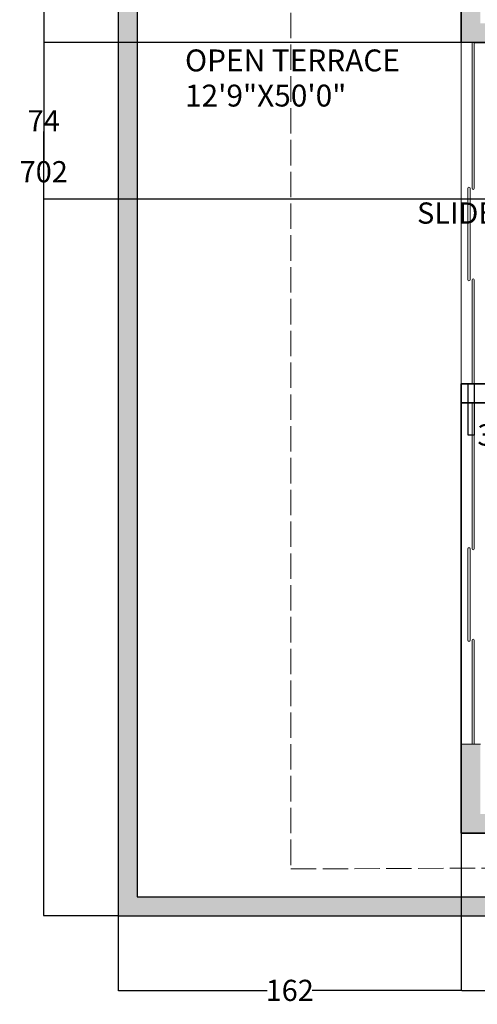
# Model space of a CAD drawing. Units: inches. Extents: x 409 to 1056, y 160 to 945.
# Tile 1 of 6: x 409 to 625, y 160 to 624. Entities that reach past the tile are written whole.
import ezdxf

# ---------------------------------------------------------------- set-up
doc = ezdxf.new("R2010")
doc.units = ezdxf.units.IN
doc.header["$MEASUREMENT"] = 0
doc.linetypes.add('ACAD_ISO02W100', pattern=[15, 12, -3])
for name, color, linetype, lineweight in [('A-ANNO-DIMS', 2, 'Continuous', 18), ('A-AREA-IDEN', 7, 'Continuous', 18), ('A-GLAZ', 4, 'Continuous', 18), ('A-ROOF-BYND', 8, 'ACAD_ISO02W100', 13), ('A-WALL', 7, 'Continuous', 35), ('A-WALL-PRPT', 7, 'Continuous', 30)]:
    doc.layers.add(name, color=color, linetype=linetype, lineweight=lineweight)
doc.layers.add('A-WALL-PATT', color=251, linetype='Continuous', lineweight=13, true_color=0x636466)
doc.styles.get("Standard").update_dxf_attribs({"font": 'arial.ttf'})
doc.dimstyles.get("Standard").update_dxf_attribs({"dimtxt": 10, "dimasz": 0.18, "dimexe": 0.18, "dimexo": 0.0625, "dimgap": 0.09, "dimtad": 0, "dimtih": 1, "dimtoh": 1, "dimdec": 0, "dimzin": 0, "dimdsep": 46, "dimlunit": 3, "dimtxsty": 'Standard', "dimcen": 0.09, "dimadec": 0, "dimazin": 0, "dimtfac": 1, "dimtdec": 0, "dimtofl": 0, "dimtmove": 0, "dimatfit": 3, "dimfxl": 1, "dimtolj": 1, "dimtzin": 0, "dimarcsym": 0})

# ---------------------------------------------------------------- blocks, each defined once
blk = doc.blocks.new('GLAZ-SLIDING-161IN')
for p, q in [((2, 161), (2, 92.18)), ((3, 161), (3, 92.18)), ((0, 92.18), (0, 49.01)), ((1, 92.18), (1, 49.01)), ((2, 49.01), (2, 0)), ((3, 49.01), (3, 0))]:
    blk.add_line(p, q)
for centre, start, end in [((0.5, 92.18), 0, 180), ((2.5, 92.18), 180, 0), ((0.5, 49.01), 180, 0), ((2.5, 49.01), 0, 180)]:
    blk.add_arc(centre, 0.5, start, end)
blk = doc.blocks.new('*D13')
at = {"layer": 'A-ANNO-DIMS', "color": 0, "lineweight": -2, "transparency": 16777216}
for p, q in [((623.91, 613.74), (648.18, 613.74)), ((648, 613.56), (648, 538.5)), ((648, 452.92), (648, 527.98)), ((623.91, 452.74), (648.18, 452.74))]:
    blk.add_line(p, q, dxfattribs=at)
at = {"layer": 'A-ANNO-DIMS', "color": 0, "transparency": 16777216}
for points in [[(647.97, 613.56), (648.03, 613.56), (648, 613.74)], [(647.97, 452.92), (648.03, 452.92), (648, 452.74)]]:
    blk.add_solid(points, dxfattribs=at)
at = {"layer": 'Defpoints', "color": 0, "transparency": 16777216}
for p in [(623.85, 613.74), (648, 613.74), (623.85, 452.74)]:
    blk.add_point(p, dxfattribs=at)
at = {"layer": 'A-ANNO-DIMS', "color": 0, "transparency": 16777216, "insert": (648, 533.24), "char_height": 10, "attachment_point": 5}
blk.add_mtext('\\A1;SLIDER 161 TYP.', dxfattribs=at)
blk = doc.blocks.new('*D14')
at = {"layer": 'A-ANNO-DIMS', "color": 0, "lineweight": -2, "transparency": 16777216}
for p, q in [((620.85, 452.68), (620.85, 428.41)), ((623.85, 452.68), (623.85, 428.41)), ((621.03, 428.59), (623.67, 428.59)), ((623.85, 428.59), (624.03, 428.59))]:
    blk.add_line(p, q, dxfattribs=at)
at = {"layer": 'A-ANNO-DIMS', "color": 0, "transparency": 16777216}
for points in [[(621.03, 428.62), (621.03, 428.56), (620.85, 428.59)], [(623.67, 428.62), (623.67, 428.56), (623.85, 428.59)]]:
    blk.add_solid(points, dxfattribs=at)
at = {"layer": 'Defpoints', "color": 0, "transparency": 16777216}
for p in [(620.85, 452.74), (623.85, 452.74), (623.85, 428.59)]:
    blk.add_point(p, dxfattribs=at)
at = {"layer": 'A-ANNO-DIMS', "color": 0, "transparency": 16777216, "insert": (644.57, 428.59), "char_height": 10, "attachment_point": 5}
blk.add_mtext('\\A1;3 TYP.', dxfattribs=at)
blk = doc.blocks.new('*D36')
at = {"layer": 'A-ANNO-DIMS', "color": 0, "lineweight": -2, "transparency": 16777216}
for p, q in [((455.68, 903.74), (420.44, 903.74)), ((420.62, 903.56), (420.62, 557.94)), ((420.62, 201.92), (420.62, 547.55)), ((455.68, 201.74), (420.44, 201.74))]:
    blk.add_line(p, q, dxfattribs=at)
at = {"layer": 'A-ANNO-DIMS', "color": 0, "transparency": 16777216}
for points in [[(420.59, 903.56), (420.65, 903.56), (420.62, 903.74)], [(420.59, 201.92), (420.65, 201.92), (420.62, 201.74)]]:
    blk.add_solid(points, dxfattribs=at)
at = {"layer": 'Defpoints', "color": 0, "transparency": 16777216}
for p in [(420.62, 903.74), (455.74, 903.74), (455.74, 201.74)]:
    blk.add_point(p, dxfattribs=at)
at = {"layer": 'A-ANNO-DIMS', "color": 0, "transparency": 16777216, "insert": (420.62, 552.74), "char_height": 10, "attachment_point": 5}
blk.add_mtext('\\A1;702', dxfattribs=at)
blk = doc.blocks.new('*D37')
at = {"layer": 'A-ANNO-DIMS', "color": 0, "lineweight": -2, "transparency": 16777216}
for p, q in [((617.74, 240.68), (617.74, 166.44)), ((971.74, 240.68), (971.74, 166.44)), ((617.92, 166.62), (783.63, 166.62)), ((971.56, 166.62), (805.85, 166.62))]:
    blk.add_line(p, q, dxfattribs=at)
at = {"layer": 'A-ANNO-DIMS', "color": 0, "transparency": 16777216}
for points in [[(617.92, 166.65), (617.92, 166.59), (617.74, 166.62)], [(971.56, 166.65), (971.56, 166.59), (971.74, 166.62)]]:
    blk.add_solid(points, dxfattribs=at)
at = {"layer": 'Defpoints', "color": 0, "transparency": 16777216}
for p in [(617.74, 240.74), (971.74, 240.74), (971.74, 166.62)]:
    blk.add_point(p, dxfattribs=at)
at = {"layer": 'A-ANNO-DIMS', "color": 0, "transparency": 16777216, "insert": (794.74, 166.62), "char_height": 10, "attachment_point": 5}
blk.add_mtext('\\A1;354', dxfattribs=at)
blk = doc.blocks.new('*D52')
at = {"layer": 'A-ANNO-DIMS', "color": 0, "lineweight": -2, "transparency": 16777216}
for p, q in [((768.679251, 613.743876), (420.436751, 613.743876)), ((420.616751, 613.563876), (420.616751, 581.833876)), ((420.616751, 539.923876), (420.616751, 571.653876)), ((768.679251, 539.743876), (420.436751, 539.743876))]:
    blk.add_line(p, q, dxfattribs=at)
at = {"layer": 'A-ANNO-DIMS', "color": 0, "transparency": 16777216}
for points in [[(420.586751, 613.563876), (420.646751, 613.563876), (420.616751, 613.743876)], [(420.586751, 539.923876), (420.646751, 539.923876), (420.616751, 539.743876)]]:
    blk.add_solid(points, dxfattribs=at)
at = {"layer": 'Defpoints', "color": 0, "transparency": 16777216}
for p in [(420.616751, 613.743876), (768.741751, 613.743876), (768.741751, 539.743876)]:
    blk.add_point(p, dxfattribs=at)
at = {"layer": 'A-ANNO-DIMS', "color": 0, "transparency": 16777216, "insert": (420.616751, 576.743876), "char_height": 10, "attachment_point": 5}
blk.add_mtext('\\A1;74', dxfattribs=at)
blk = doc.blocks.new('*D58')
at = {"layer": 'A-ANNO-DIMS', "color": 0, "lineweight": -2, "transparency": 16777216}
for p, q in [((617.74, 240.68), (617.74, 166.44)), ((455.74, 201.68), (455.74, 166.44)), ((455.92, 166.62), (526.13, 166.62)), ((617.56, 166.62), (547.36, 166.62))]:
    blk.add_line(p, q, dxfattribs=at)
at = {"layer": 'A-ANNO-DIMS', "color": 0, "transparency": 16777216}
for points in [[(455.92, 166.65), (455.92, 166.59), (455.74, 166.62)], [(617.56, 166.65), (617.56, 166.59), (617.74, 166.62)]]:
    blk.add_solid(points, dxfattribs=at)
at = {"layer": 'Defpoints', "color": 0, "transparency": 16777216}
for p in [(617.74, 240.74), (455.74, 201.74), (617.74, 166.62)]:
    blk.add_point(p, dxfattribs=at)
at = {"layer": 'A-ANNO-DIMS', "color": 0, "transparency": 16777216, "insert": (536.74, 166.62), "char_height": 10, "attachment_point": 5}
blk.add_mtext('\\A1;162', dxfattribs=at)

msp = doc.modelspace()

# ---------------------------------------------------------------- hatches: boundary and pattern name
at = {"layer": 'A-WALL-PATT'}
h = msp.add_hatch(color=256, dxfattribs=at)
h.dxf.hatch_style = 1
h.paths.add_polyline_path([(730.4481, 698.1956), (696.9841, 709.3369, 1), (696.9841, 678.8752)], flags=17)
h.paths.add_polyline_path([(803.8768, 698.1956), (770.4128, 709.3369, 1), (770.4128, 678.8752)], flags=17)
h.paths.add_polyline_path([(464.7418, 894.7439), (466.7418, 894.7439), (962.7418, 894.7439), (962.7418, 810.7439), (971.7418, 810.7439), (971.7418, 903.7439), (455.7418, 903.7439), (455.7418, 201.7439), (971.7418, 201.7439), (971.7418, 240.7439), (962.7418, 240.7439), (962.7418, 210.7439), (464.7418, 210.7439)])
h = msp.add_hatch(color=256, dxfattribs=at)
h.dxf.hatch_style = 1
h.paths.add_polyline_path([(626.7418, 801.7439), (870.7418, 801.7439), (870.7418, 710.7439), (870.7418, 683.9043), (875.7418, 683.9043), (875.7418, 707.7439), (962.7418, 707.7439), (962.7418, 710.7439), (875.7418, 710.7439), (875.7418, 722.7439), (875.7418, 801.7439), (885.6955, 801.7439, -0.06325422), (884.5523, 810.7439), (617.7418, 810.7439), (617.7418, 732.9297), (626.7418, 732.9297)])
h.paths.add_polyline_path([(962.7418, 810.7439), (920.5523, 810.7439), (920.5523, 801.7439), (962.7418, 801.7439)], flags=17)
h.paths.add_polyline_path([(971.7418, 810.7439), (962.7418, 810.7439), (962.7418, 801.7439), (962.7418, 707.7439), (962.7418, 622.7439), (962.7418, 613.7439), (962.7418, 548.7439), (856.7418, 548.7439), (847.7418, 548.7439), (776.7418, 548.7439), (776.7418, 569.8172), (768.7418, 569.8172), (768.7418, 539.7439), (847.7418, 539.7439), (971.7418, 539.7439), (971.7418, 613.7439), (971.7418, 707.7439)])
h.paths.add_polyline_path([(883.2418, 622.7439), (875.7418, 622.7439), (684.4993, 622.7439, -0.06325422), (685.6424, 613.7439), (870.7418, 613.7439), (875.7418, 613.7439), (884.3849, 613.7439, -0.06325422)])
h.paths.add_polyline_path([(649.6424, 622.7439), (626.7418, 622.7439), (626.7418, 613.7439), (649.6424, 613.7439)])
h.paths.add_polyline_path([(626.7418, 652.3165), (617.7418, 652.3165), (617.7418, 613.7439), (626.7418, 613.7439), (626.7418, 622.7439)])
h.paths.add_polyline_path([(776.7418, 613.7439), (768.7418, 613.7439), (768.7418, 590.4138), (776.7418, 590.4138)], flags=17)
h.paths.add_polyline_path([(856.7418, 613.7439), (847.7418, 613.7439), (847.7418, 548.7439), (856.7418, 548.7439)], flags=17)
h.paths.add_polyline_path([(962.7418, 622.7439), (919.2418, 622.7439), (919.2418, 613.7439), (962.7418, 613.7439)], flags=17)
h.paths.add_polyline_path([(971.7418, 539.7439), (962.7418, 539.7439), (962.7418, 452.7439), (687.1506, 452.7439, -0.06325422), (686.0074, 443.7439), (962.7418, 443.7439), (962.7418, 331.7439), (927.6873, 331.7439, -0.02784244), (927.9102, 327.7439), (962.7418, 327.7439), (962.7418, 249.7439), (871.7418, 249.7439), (870.7418, 249.7439), (626.7418, 249.7439), (626.7418, 282.7439), (617.7418, 282.7439), (617.7418, 240.7439), (870.7418, 240.7439), (871.7418, 240.7439), (971.7418, 240.7439), (971.7418, 249.7439), (971.7418, 327.7439), (971.7418, 331.7439), (971.7418, 443.7439), (971.7418, 452.7439)])
h.paths.add_polyline_path([(875.7418, 443.7439), (870.7418, 443.7439), (870.7418, 327.7439), (871.7418, 327.7439), (891.9102, 327.7439), (891.9102, 331.7439), (875.7418, 331.7439)], flags=17)

# ---------------------------------------------------------------- linework, layer by layer
at = {"layer": 'A-GLAZ'}
for p, q in [((617.7418, 613.7439), (617.7418, 452.7439)), ((626.7418, 613.7439), (617.7418, 613.7439)), ((623.8487, 282.7439), (617.7418, 282.7439)), ((617.7418, 282.7439), (626.7418, 282.7439))]:
    msp.add_line(p, q, dxfattribs=at)
at = {"layer": 'A-ROOF-BYND'}
for p, q in [((537.2978, 852.7439), (537.2978, 223.8898)), ((537.2978, 223.8898), (962.7418, 225.7439))]:
    msp.add_line(p, q, dxfattribs=at)
at = {"layer": 'A-WALL'}
for p, q in [((617.7418, 810.7439), (617.7418, 613.7439)), ((617.7418, 452.7439), (962.7418, 452.7439)), ((617.7418, 443.7439), (617.7418, 452.7439)), ((617.7418, 443.7439), (652.1506, 443.7439)), ((617.7418, 443.7439), (617.7418, 240.7439)), ((617.7418, 240.7439), (870.7418, 240.7439))]:
    msp.add_line(p, q, dxfattribs=at)
at = {"layer": 'A-WALL-PRPT'}
for p, q in [((455.7418, 903.7439), (455.7418, 201.7439)), ((464.7418, 894.7439), (464.7418, 210.7439)), ((464.7418, 210.7439), (962.7418, 210.7439)), ((455.7418, 201.7439), (971.7418, 201.7439))]:
    msp.add_line(p, q, dxfattribs=at)

# ---------------------------------------------------------------- block references
at = {"layer": 'A-GLAZ'}
for p in [(620.849, 452.744), (620.849, 282.744)]:
    msp.add_blockref('GLAZ-SLIDING-161IN', p, dxfattribs=at)

# ---------------------------------------------------------------- texts
at = {"layer": 'A-AREA-IDEN'}
for s, p in [('OPEN TERRACE ', (487.3011, 600.0713)), ('12\'9"X50\'0"', (487.3011, 583.4838))]:
    msp.add_text(s, height=10.325829, dxfattribs=at).set_placement(p)

# ---------------------------------------------------------------- dimensions: what is measured, and where the dimension line sits
at = {"layer": 'A-ANNO-DIMS'}
for base, p1, p2, picture, middle in [((420.6168, 903.7439), (455.7418, 201.7439), (455.7418, 903.7439), '*D36', (420.6168, 552.7439)), ((420.6168, 613.7439), (768.7418, 539.7439), (768.7418, 613.7439), '*D52', (420.6168, 576.7439))]:
    dim = msp.add_linear_dim(base=base, p1=p1, p2=p2, angle=90, dimstyle='Standard', override={"dimdec": 0, "dimlfac": 1, "dimrnd": 0, "dimzin": 0, "dimdsep": 46, "dimlunit": 2}, dxfattribs=at)
    dim.commit()
    dim.dimension.update_dxf_attribs({"geometry": picture, "text_midpoint": middle})
dim = msp.add_linear_dim(base=(647.9987, 613.7439), p1=(623.8487, 452.7439), p2=(623.8487, 613.7439), angle=90, text='SLIDER <> TYP.', dimstyle='Standard', override={"dimdec": 0, "dimlfac": 1, "dimrnd": 0, "dimzin": 0, "dimdsep": 46, "dimlunit": 2}, dxfattribs=at)
dim.commit()
dim.dimension.update_dxf_attribs({"geometry": '*D13', "text_midpoint": (647.9987, 533.2439)})
dim = msp.add_linear_dim(base=(623.8487, 428.5939), p1=(620.8487, 452.7439), p2=(623.8487, 452.7439), text='<> TYP.', dimstyle='Standard', override={"dimdec": 0, "dimlfac": 1, "dimrnd": 0, "dimzin": 0, "dimdsep": 46, "dimlunit": 2}, dxfattribs=at)
dim.commit()
dim.dimension.update_dxf_attribs({"geometry": '*D14', "text_midpoint": (644.5689, 428.5939)})
for base, p1, p2, picture, middle in [((617.7418, 166.6189), (455.7418, 201.7439), (617.7418, 240.7439), '*D58', (536.7418, 166.6189)), ((971.7418, 166.6189), (617.7418, 240.7439), (971.7418, 240.7439), '*D37', (794.7418, 166.6189))]:
    dim = msp.add_linear_dim(base=base, p1=p1, p2=p2, dimstyle='Standard', override={"dimdec": 0, "dimlfac": 1, "dimrnd": 0, "dimzin": 0, "dimdsep": 46, "dimlunit": 2}, dxfattribs=at)
    dim.commit()
    dim.dimension.update_dxf_attribs({"geometry": picture, "text_midpoint": middle})

doc.saveas('drawing.dxf')
